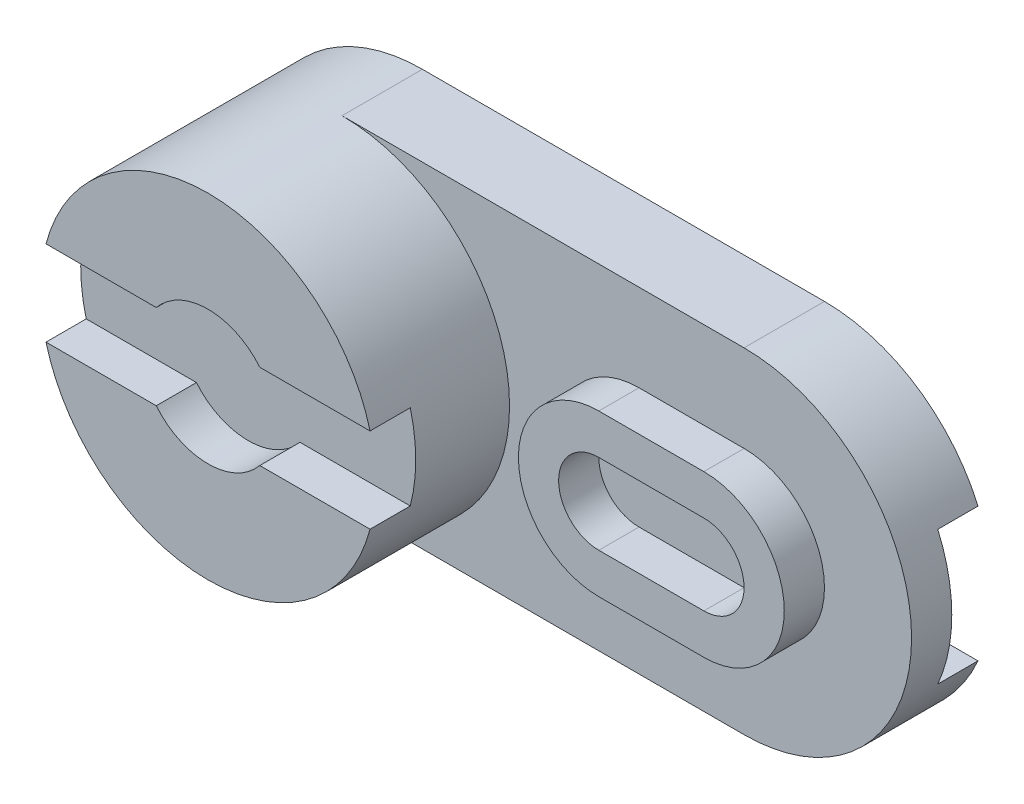
ISO-10303-21;
HEADER;
FILE_DESCRIPTION(('STEP AP214'),'2;1');
FILE_NAME('part.step','',(''),(''),'','','');
FILE_SCHEMA(('AUTOMOTIVE_DESIGN { 1 0 10303 214 1 1 1 1 }'));
ENDSEC;
DATA;
#1=APPLICATION_CONTEXT('core data for automotive mechanical design processes');
#2=APPLICATION_PROTOCOL_DEFINITION('international standard','automotive_design',2000,#1);
#3=PRODUCT_CONTEXT('',#1,'mechanical');
#4=PRODUCT('Part','Part','',(#3));
#5=PRODUCT_RELATED_PRODUCT_CATEGORY('part','',(#4));
#6=PRODUCT_DEFINITION_FORMATION('','',#4);
#7=PRODUCT_DEFINITION_CONTEXT('part definition',#1,'design');
#8=PRODUCT_DEFINITION('design','',#6,#7);
#9=PRODUCT_DEFINITION_SHAPE('','',#8);
#10=(LENGTH_UNIT() NAMED_UNIT(*) SI_UNIT(.MILLI.,.METRE.));
#11=(NAMED_UNIT(*) PLANE_ANGLE_UNIT() SI_UNIT($,.RADIAN.));
#12=(NAMED_UNIT(*) SI_UNIT($,.STERADIAN.) SOLID_ANGLE_UNIT());
#13=UNCERTAINTY_MEASURE_WITH_UNIT(LENGTH_MEASURE(1.E-05),#10,'distance_accuracy_value','');
#14=(GEOMETRIC_REPRESENTATION_CONTEXT(3) GLOBAL_UNCERTAINTY_ASSIGNED_CONTEXT((#13)) GLOBAL_UNIT_ASSIGNED_CONTEXT((#10,
#11,#12)) REPRESENTATION_CONTEXT('',''));
#15=CARTESIAN_POINT('',(0.,0.,0.));
#16=DIRECTION('',(0.,0.,1.));
#17=DIRECTION('',(1.,0.,0.));
#18=AXIS2_PLACEMENT_3D('',#15,#16,#17);
#19=CARTESIAN_POINT('',(0.,0.,12.));
#20=DIRECTION('',(0.,0.,1.));
#21=DIRECTION('',(1.,0.,0.));
#22=AXIS2_PLACEMENT_3D('',#19,#20,#21);
#23=PLANE('',#22);
#24=CARTESIAN_POINT('',(0.,0.,12.));
#25=DIRECTION('',(0.,0.,1.));
#26=DIRECTION('',(1.,0.,0.));
#27=AXIS2_PLACEMENT_3D('',#24,#25,#26);
#28=CIRCLE('',#27,25.);
#29=CARTESIAN_POINT('',(0.,-25.,12.));
#30=VERTEX_POINT('',#29);
#31=CARTESIAN_POINT('',(0.,25.,12.));
#32=VERTEX_POINT('',#31);
#33=EDGE_CURVE('E348',#30,#32,#28,.T.);
#34=ORIENTED_EDGE('',*,*,#33,.F.);
#35=DIRECTION('',(1.,0.,0.));
#36=VECTOR('',#35,1.);
#37=CARTESIAN_POINT('',(0.,-25.,12.));
#38=LINE('',#37,#36);
#39=CARTESIAN_POINT('',(60.,-25.,12.));
#40=VERTEX_POINT('',#39);
#41=EDGE_CURVE('E353',#30,#40,#38,.T.);
#42=ORIENTED_EDGE('',*,*,#41,.T.);
#43=CARTESIAN_POINT('',(60.,0.,12.));
#44=DIRECTION('',(0.,0.,1.));
#45=DIRECTION('',(1.,0.,0.));
#46=AXIS2_PLACEMENT_3D('',#43,#44,#45);
#47=CIRCLE('',#46,25.);
#48=CARTESIAN_POINT('',(60.,25.,12.));
#49=VERTEX_POINT('',#48);
#50=EDGE_CURVE('E359',#40,#49,#47,.T.);
#51=ORIENTED_EDGE('',*,*,#50,.T.);
#52=DIRECTION('',(-1.,0.,0.));
#53=VECTOR('',#52,1.);
#54=CARTESIAN_POINT('',(0.,25.,12.));
#55=LINE('',#54,#53);
#56=EDGE_CURVE('E356',#49,#32,#55,.T.);
#57=ORIENTED_EDGE('',*,*,#56,.T.);
#58=EDGE_LOOP('',(#34,#42,#51,#57));
#59=FACE_BOUND('',#58,.T.);
#60=DIRECTION('',(1.,0.,0.));
#61=VECTOR('',#60,1.);
#62=CARTESIAN_POINT('',(44.3230167016828,-12.,12.));
#63=LINE('',#62,#61);
#64=CARTESIAN_POINT('',(44.3230167016828,-12.,12.));
#65=VERTEX_POINT('',#64);
#66=CARTESIAN_POINT('',(60.,-12.,12.));
#67=VERTEX_POINT('',#66);
#68=EDGE_CURVE('E276',#65,#67,#63,.T.);
#69=ORIENTED_EDGE('',*,*,#68,.F.);
#70=CARTESIAN_POINT('',(44.3230167016828,0.,12.));
#71=DIRECTION('',(0.,0.,1.));
#72=DIRECTION('',(1.,0.,0.));
#73=AXIS2_PLACEMENT_3D('',#70,#71,#72);
#74=CIRCLE('',#73,12.);
#75=CARTESIAN_POINT('',(44.3230167016828,12.,12.));
#76=VERTEX_POINT('',#75);
#77=EDGE_CURVE('E264',#76,#65,#74,.T.);
#78=ORIENTED_EDGE('',*,*,#77,.F.);
#79=DIRECTION('',(-1.,0.,0.));
#80=VECTOR('',#79,1.);
#81=CARTESIAN_POINT('',(44.3230167016828,12.,12.));
#82=LINE('',#81,#80);
#83=CARTESIAN_POINT('',(60.,12.,12.));
#84=VERTEX_POINT('',#83);
#85=EDGE_CURVE('E269',#84,#76,#82,.T.);
#86=ORIENTED_EDGE('',*,*,#85,.F.);
#87=CARTESIAN_POINT('',(60.,0.,12.));
#88=DIRECTION('',(0.,0.,1.));
#89=DIRECTION('',(1.,0.,0.));
#90=AXIS2_PLACEMENT_3D('',#87,#88,#89);
#91=CIRCLE('',#90,12.);
#92=EDGE_CURVE('E282',#67,#84,#91,.T.);
#93=ORIENTED_EDGE('',*,*,#92,.F.);
#94=EDGE_LOOP('',(#69,#78,#86,#93));
#95=FACE_BOUND('',#94,.T.);
#96=ADVANCED_FACE('F39',(#59,#95),#23,.T.);
#97=CARTESIAN_POINT('',(0.,0.,12.));
#98=DIRECTION('',(0.,0.,-1.));
#99=DIRECTION('',(-1.,0.,0.));
#100=AXIS2_PLACEMENT_3D('',#97,#98,#99);
#101=CYLINDRICAL_SURFACE('',#100,25.);
#102=CARTESIAN_POINT('',(0.,0.,0.));
#103=DIRECTION('',(0.,0.,1.));
#104=DIRECTION('',(1.,0.,0.));
#105=AXIS2_PLACEMENT_3D('',#102,#103,#104);
#106=CIRCLE('',#105,25.);
#107=CARTESIAN_POINT('',(0.,25.,0.));
#108=VERTEX_POINT('',#107);
#109=CARTESIAN_POINT('',(0.,-25.,0.));
#110=VERTEX_POINT('',#109);
#111=EDGE_CURVE('E349',#108,#110,#106,.T.);
#112=ORIENTED_EDGE('',*,*,#111,.T.);
#113=DIRECTION('',(0.,0.,-1.));
#114=VECTOR('',#113,1.);
#115=CARTESIAN_POINT('',(0.,-25.,12.));
#116=LINE('',#115,#114);
#117=EDGE_CURVE('E351',#30,#110,#116,.T.);
#118=ORIENTED_EDGE('',*,*,#117,.F.);
#119=ORIENTED_EDGE('',*,*,#33,.T.);
#120=DIRECTION('',(0.,0.,-1.));
#121=VECTOR('',#120,1.);
#122=CARTESIAN_POINT('',(0.,25.,12.));
#123=LINE('',#122,#121);
#124=EDGE_CURVE('E361',#32,#108,#123,.T.);
#125=ORIENTED_EDGE('',*,*,#124,.T.);
#126=EDGE_LOOP('',(#112,#118,#119,#125));
#127=FACE_BOUND('',#126,.T.);
#128=DIRECTION('',(0.,0.,1.));
#129=VECTOR('',#128,1.);
#130=CARTESIAN_POINT('',(-24.1806910636993,-6.34776966200989,26.));
#131=LINE('',#130,#129);
#132=CARTESIAN_POINT('',(-24.1806910636993,-6.34776966200989,26.));
#133=VERTEX_POINT('',#132);
#134=CARTESIAN_POINT('',(-24.1806910636993,-6.34776966200989,32.));
#135=VERTEX_POINT('',#134);
#136=EDGE_CURVE('E330',#133,#135,#131,.T.);
#137=ORIENTED_EDGE('',*,*,#136,.F.);
#138=CARTESIAN_POINT('',(0.,0.,26.));
#139=DIRECTION('',(0.,0.,1.));
#140=DIRECTION('',(1.,0.,0.));
#141=AXIS2_PLACEMENT_3D('',#138,#139,#140);
#142=CIRCLE('',#141,25.);
#143=CARTESIAN_POINT('',(-24.1806910636993,6.34776966200989,26.));
#144=VERTEX_POINT('',#143);
#145=EDGE_CURVE('E313',#144,#133,#142,.T.);
#146=ORIENTED_EDGE('',*,*,#145,.F.);
#147=DIRECTION('',(0.,0.,1.));
#148=VECTOR('',#147,1.);
#149=CARTESIAN_POINT('',(-24.1806910636993,6.34776966200989,26.));
#150=LINE('',#149,#148);
#151=CARTESIAN_POINT('',(-24.1806910636993,6.34776966200989,32.));
#152=VERTEX_POINT('',#151);
#153=EDGE_CURVE('E329',#144,#152,#150,.T.);
#154=ORIENTED_EDGE('',*,*,#153,.T.);
#155=CARTESIAN_POINT('',(0.,0.,32.));
#156=DIRECTION('',(0.,0.,1.));
#157=DIRECTION('',(1.,0.,0.));
#158=AXIS2_PLACEMENT_3D('',#155,#156,#157);
#159=CIRCLE('',#158,25.);
#160=CARTESIAN_POINT('',(24.1806910636993,6.34776966200989,32.));
#161=VERTEX_POINT('',#160);
#162=EDGE_CURVE('E347',#161,#152,#159,.T.);
#163=ORIENTED_EDGE('',*,*,#162,.F.);
#164=DIRECTION('',(0.,0.,1.));
#165=VECTOR('',#164,1.);
#166=CARTESIAN_POINT('',(24.1806910636993,6.34776966200989,26.));
#167=LINE('',#166,#165);
#168=CARTESIAN_POINT('',(24.1806910636993,6.34776966200989,26.));
#169=VERTEX_POINT('',#168);
#170=EDGE_CURVE('E339',#169,#161,#167,.T.);
#171=ORIENTED_EDGE('',*,*,#170,.F.);
#172=CARTESIAN_POINT('',(0.,0.,26.));
#173=DIRECTION('',(0.,0.,1.));
#174=DIRECTION('',(1.,0.,0.));
#175=AXIS2_PLACEMENT_3D('',#172,#173,#174);
#176=CIRCLE('',#175,25.);
#177=CARTESIAN_POINT('',(24.1806910636993,-6.34776966200989,26.));
#178=VERTEX_POINT('',#177);
#179=EDGE_CURVE('E302',#178,#169,#176,.T.);
#180=ORIENTED_EDGE('',*,*,#179,.F.);
#181=DIRECTION('',(0.,0.,1.));
#182=VECTOR('',#181,1.);
#183=CARTESIAN_POINT('',(24.1806910636993,-6.34776966200989,26.));
#184=LINE('',#183,#182);
#185=CARTESIAN_POINT('',(24.1806910636993,-6.34776966200989,32.));
#186=VERTEX_POINT('',#185);
#187=EDGE_CURVE('E336',#178,#186,#184,.T.);
#188=ORIENTED_EDGE('',*,*,#187,.T.);
#189=EDGE_CURVE('E328',#135,#186,#159,.T.);
#190=ORIENTED_EDGE('',*,*,#189,.F.);
#191=EDGE_LOOP('',(#137,#146,#154,#163,#171,#180,#188,#190));
#192=FACE_BOUND('',#191,.T.);
#193=ADVANCED_FACE('F41',(#127,#192),#101,.T.);
#194=CARTESIAN_POINT('',(0.,0.,32.));
#195=DIRECTION('',(0.,0.,1.));
#196=DIRECTION('',(1.,0.,0.));
#197=AXIS2_PLACEMENT_3D('',#194,#195,#196);
#198=PLANE('',#197);
#199=CARTESIAN_POINT('',(0.,0.,32.));
#200=DIRECTION('',(0.,0.,1.));
#201=DIRECTION('',(1.,0.,0.));
#202=AXIS2_PLACEMENT_3D('',#199,#200,#201);
#203=CIRCLE('',#202,10.);
#204=CARTESIAN_POINT('',(-7.72695414235563,-6.34776966200989,32.));
#205=VERTEX_POINT('',#204);
#206=CARTESIAN_POINT('',(7.72695414235563,-6.34776966200989,32.));
#207=VERTEX_POINT('',#206);
#208=EDGE_CURVE('E320',#205,#207,#203,.T.);
#209=ORIENTED_EDGE('',*,*,#208,.F.);
#210=DIRECTION('',(-1.,0.,0.));
#211=VECTOR('',#210,1.);
#212=CARTESIAN_POINT('',(0.,-6.34776966200989,32.));
#213=LINE('',#212,#211);
#214=EDGE_CURVE('E295',#205,#135,#213,.T.);
#215=ORIENTED_EDGE('',*,*,#214,.T.);
#216=ORIENTED_EDGE('',*,*,#189,.T.);
#217=DIRECTION('',(1.,0.,0.));
#218=VECTOR('',#217,1.);
#219=CARTESIAN_POINT('',(0.,-6.34776966200989,32.));
#220=LINE('',#219,#218);
#221=EDGE_CURVE('E319',#207,#186,#220,.T.);
#222=ORIENTED_EDGE('',*,*,#221,.F.);
#223=EDGE_LOOP('',(#209,#215,#216,#222));
#224=FACE_BOUND('',#223,.T.);
#225=ADVANCED_FACE('F427',(#224),#198,.T.);
#226=CARTESIAN_POINT('',(0.,-25.,12.));
#227=DIRECTION('',(0.,1.,0.));
#228=DIRECTION('',(-1.,0.,0.));
#229=AXIS2_PLACEMENT_3D('',#226,#227,#228);
#230=PLANE('',#229);
#231=DIRECTION('',(1.,0.,0.));
#232=VECTOR('',#231,1.);
#233=CARTESIAN_POINT('',(0.,-25.,0.));
#234=LINE('',#233,#232);
#235=CARTESIAN_POINT('',(60.,-25.,0.));
#236=VERTEX_POINT('',#235);
#237=EDGE_CURVE('E368',#110,#236,#234,.T.);
#238=ORIENTED_EDGE('',*,*,#237,.T.);
#239=DIRECTION('',(0.,0.,-1.));
#240=VECTOR('',#239,1.);
#241=CARTESIAN_POINT('',(60.,-25.,12.));
#242=LINE('',#241,#240);
#243=EDGE_CURVE('E381',#40,#236,#242,.T.);
#244=ORIENTED_EDGE('',*,*,#243,.F.);
#245=ORIENTED_EDGE('',*,*,#41,.F.);
#246=ORIENTED_EDGE('',*,*,#117,.T.);
#247=EDGE_LOOP('',(#238,#244,#245,#246));
#248=FACE_BOUND('',#247,.T.);
#249=ADVANCED_FACE('F402',(#248),#230,.F.);
#250=CARTESIAN_POINT('',(60.,0.,12.));
#251=DIRECTION('',(0.,0.,-1.));
#252=DIRECTION('',(-1.,0.,0.));
#253=AXIS2_PLACEMENT_3D('',#250,#251,#252);
#254=CYLINDRICAL_SURFACE('',#253,25.);
#255=CARTESIAN_POINT('',(60.,0.,6.));
#256=DIRECTION('',(0.,0.,-1.));
#257=DIRECTION('',(-1.,0.,0.));
#258=AXIS2_PLACEMENT_3D('',#255,#256,#257);
#259=CIRCLE('',#258,25.);
#260=CARTESIAN_POINT('',(82.9128784747792,10.,6.));
#261=VERTEX_POINT('',#260);
#262=CARTESIAN_POINT('',(82.9128784747792,-10.,6.));
#263=VERTEX_POINT('',#262);
#264=EDGE_CURVE('E225',#261,#263,#259,.T.);
#265=ORIENTED_EDGE('',*,*,#264,.F.);
#266=DIRECTION('',(0.,0.,-1.));
#267=VECTOR('',#266,1.);
#268=CARTESIAN_POINT('',(82.9128784747792,10.,6.));
#269=LINE('',#268,#267);
#270=CARTESIAN_POINT('',(82.9128784747792,10.,-6.E-06));
#271=VERTEX_POINT('',#270);
#272=EDGE_CURVE('E218',#261,#271,#269,.T.);
#273=ORIENTED_EDGE('',*,*,#272,.T.);
#274=CARTESIAN_POINT('',(60.,0.,0.));
#275=DIRECTION('',(0.,0.,1.));
#276=DIRECTION('',(1.,0.,0.));
#277=AXIS2_PLACEMENT_3D('',#274,#275,#276);
#278=CIRCLE('',#277,25.);
#279=CARTESIAN_POINT('',(60.,25.,0.));
#280=VERTEX_POINT('',#279);
#281=EDGE_CURVE('E366',#271,#280,#278,.T.);
#282=ORIENTED_EDGE('',*,*,#281,.T.);
#283=DIRECTION('',(0.,0.,-1.));
#284=VECTOR('',#283,1.);
#285=CARTESIAN_POINT('',(60.,25.,12.));
#286=LINE('',#285,#284);
#287=EDGE_CURVE('E383',#49,#280,#286,.T.);
#288=ORIENTED_EDGE('',*,*,#287,.F.);
#289=ORIENTED_EDGE('',*,*,#50,.F.);
#290=ORIENTED_EDGE('',*,*,#243,.T.);
#291=CARTESIAN_POINT('',(82.9128784747792,-10.,0.));
#292=VERTEX_POINT('',#291);
#293=EDGE_CURVE('E376',#236,#292,#278,.T.);
#294=ORIENTED_EDGE('',*,*,#293,.T.);
#295=DIRECTION('',(0.,0.,-1.));
#296=VECTOR('',#295,1.);
#297=CARTESIAN_POINT('',(82.9128784747792,-10.,6.));
#298=LINE('',#297,#296);
#299=EDGE_CURVE('E54',#263,#292,#298,.T.);
#300=ORIENTED_EDGE('',*,*,#299,.F.);
#301=EDGE_LOOP('',(#265,#273,#282,#288,#289,#290,#294,#300));
#302=FACE_BOUND('',#301,.T.);
#303=ADVANCED_FACE('F410',(#302),#254,.T.);
#304=CARTESIAN_POINT('',(0.,25.,12.));
#305=DIRECTION('',(0.,-1.,0.));
#306=DIRECTION('',(1.,0.,0.));
#307=AXIS2_PLACEMENT_3D('',#304,#305,#306);
#308=PLANE('',#307);
#309=DIRECTION('',(-1.,0.,0.));
#310=VECTOR('',#309,1.);
#311=CARTESIAN_POINT('',(0.,25.,0.));
#312=LINE('',#311,#310);
#313=EDGE_CURVE('E357',#280,#108,#312,.T.);
#314=ORIENTED_EDGE('',*,*,#313,.T.);
#315=ORIENTED_EDGE('',*,*,#124,.F.);
#316=ORIENTED_EDGE('',*,*,#56,.F.);
#317=ORIENTED_EDGE('',*,*,#287,.T.);
#318=EDGE_LOOP('',(#314,#315,#316,#317));
#319=FACE_BOUND('',#318,.T.);
#320=ADVANCED_FACE('F407',(#319),#308,.F.);
#321=CARTESIAN_POINT('',(0.,0.,0.));
#322=DIRECTION('',(0.,0.,1.));
#323=DIRECTION('',(1.,0.,0.));
#324=AXIS2_PLACEMENT_3D('',#321,#322,#323);
#325=PLANE('',#324);
#326=ORIENTED_EDGE('',*,*,#281,.F.);
#327=DIRECTION('',(-1.,0.,0.));
#328=VECTOR('',#327,1.);
#329=CARTESIAN_POINT('',(0.,10.,0.));
#330=LINE('',#329,#328);
#331=CARTESIAN_POINT('',(60.,10.,0.));
#332=VERTEX_POINT('',#331);
#333=EDGE_CURVE('E11',#271,#332,#330,.T.);
#334=ORIENTED_EDGE('',*,*,#333,.T.);
#335=DIRECTION('',(0.,-1.,0.));
#336=VECTOR('',#335,1.);
#337=CARTESIAN_POINT('',(60.,0.,0.));
#338=LINE('',#337,#336);
#339=CARTESIAN_POINT('',(60.,-10.,0.));
#340=VERTEX_POINT('',#339);
#341=EDGE_CURVE('E48',#332,#340,#338,.T.);
#342=ORIENTED_EDGE('',*,*,#341,.T.);
#343=DIRECTION('',(-1.,0.,0.));
#344=VECTOR('',#343,1.);
#345=CARTESIAN_POINT('',(0.,-10.,0.));
#346=LINE('',#345,#344);
#347=EDGE_CURVE('E355',#292,#340,#346,.T.);
#348=ORIENTED_EDGE('',*,*,#347,.F.);
#349=ORIENTED_EDGE('',*,*,#293,.F.);
#350=ORIENTED_EDGE('',*,*,#237,.F.);
#351=ORIENTED_EDGE('',*,*,#111,.F.);
#352=ORIENTED_EDGE('',*,*,#313,.F.);
#353=EDGE_LOOP('',(#326,#334,#342,#348,#349,#350,#351,#352));
#354=FACE_BOUND('',#353,.T.);
#355=ADVANCED_FACE('F398',(#354),#325,.F.);
#356=DIRECTION('',(-1.,0.,0.));
#357=VECTOR('',#356,1.);
#358=CARTESIAN_POINT('',(0.,6.34776966200989,32.));
#359=LINE('',#358,#357);
#360=CARTESIAN_POINT('',(-7.72695414235563,6.34776966200989,32.));
#361=VERTEX_POINT('',#360);
#362=EDGE_CURVE('E297',#361,#152,#359,.T.);
#363=ORIENTED_EDGE('',*,*,#362,.F.);
#364=CARTESIAN_POINT('',(7.72695414235563,6.34776966200989,32.));
#365=VERTEX_POINT('',#364);
#366=EDGE_CURVE('E321',#365,#361,#203,.T.);
#367=ORIENTED_EDGE('',*,*,#366,.F.);
#368=DIRECTION('',(1.,0.,0.));
#369=VECTOR('',#368,1.);
#370=CARTESIAN_POINT('',(0.,6.34776966200989,32.));
#371=LINE('',#370,#369);
#372=EDGE_CURVE('E323',#365,#161,#371,.T.);
#373=ORIENTED_EDGE('',*,*,#372,.T.);
#374=ORIENTED_EDGE('',*,*,#162,.T.);
#375=EDGE_LOOP('',(#363,#367,#373,#374));
#376=FACE_BOUND('',#375,.T.);
#377=ADVANCED_FACE('F506',(#376),#198,.T.);
#378=CARTESIAN_POINT('',(0.,-6.34776966200989,26.));
#379=DIRECTION('',(0.,1.,0.));
#380=DIRECTION('',(-1.,0.,0.));
#381=AXIS2_PLACEMENT_3D('',#378,#379,#380);
#382=PLANE('',#381);
#383=ORIENTED_EDGE('',*,*,#214,.F.);
#384=DIRECTION('',(0.,0.,1.));
#385=VECTOR('',#384,1.);
#386=CARTESIAN_POINT('',(-7.72695414235563,-6.34776966200989,26.));
#387=LINE('',#386,#385);
#388=CARTESIAN_POINT('',(-7.72695414235563,-6.34776966200989,26.));
#389=VERTEX_POINT('',#388);
#390=EDGE_CURVE('E314',#389,#205,#387,.T.);
#391=ORIENTED_EDGE('',*,*,#390,.F.);
#392=DIRECTION('',(-1.,0.,0.));
#393=VECTOR('',#392,1.);
#394=CARTESIAN_POINT('',(0.,-6.34776966200989,26.));
#395=LINE('',#394,#393);
#396=EDGE_CURVE('E291',#389,#133,#395,.T.);
#397=ORIENTED_EDGE('',*,*,#396,.T.);
#398=ORIENTED_EDGE('',*,*,#136,.T.);
#399=EDGE_LOOP('',(#383,#391,#397,#398));
#400=FACE_BOUND('',#399,.T.);
#401=ADVANCED_FACE('F497',(#400),#382,.T.);
#402=CARTESIAN_POINT('',(0.,6.34776966200989,26.));
#403=DIRECTION('',(0.,1.,0.));
#404=DIRECTION('',(-1.,0.,0.));
#405=AXIS2_PLACEMENT_3D('',#402,#403,#404);
#406=PLANE('',#405);
#407=ORIENTED_EDGE('',*,*,#362,.T.);
#408=ORIENTED_EDGE('',*,*,#153,.F.);
#409=DIRECTION('',(-1.,0.,0.));
#410=VECTOR('',#409,1.);
#411=CARTESIAN_POINT('',(0.,6.34776966200989,26.));
#412=LINE('',#411,#410);
#413=CARTESIAN_POINT('',(-7.72695414235563,6.34776966200989,26.));
#414=VERTEX_POINT('',#413);
#415=EDGE_CURVE('E306',#414,#144,#412,.T.);
#416=ORIENTED_EDGE('',*,*,#415,.F.);
#417=DIRECTION('',(0.,0.,1.));
#418=VECTOR('',#417,1.);
#419=CARTESIAN_POINT('',(-7.72695414235563,6.34776966200989,26.));
#420=LINE('',#419,#418);
#421=EDGE_CURVE('E334',#414,#361,#420,.T.);
#422=ORIENTED_EDGE('',*,*,#421,.T.);
#423=EDGE_LOOP('',(#407,#408,#416,#422));
#424=FACE_BOUND('',#423,.T.);
#425=ADVANCED_FACE('F495',(#424),#406,.F.);
#426=CARTESIAN_POINT('',(0.,0.,26.));
#427=DIRECTION('',(0.,0.,1.));
#428=DIRECTION('',(1.,0.,0.));
#429=AXIS2_PLACEMENT_3D('',#426,#427,#428);
#430=CYLINDRICAL_SURFACE('',#429,10.);
#431=ORIENTED_EDGE('',*,*,#366,.T.);
#432=ORIENTED_EDGE('',*,*,#421,.F.);
#433=CARTESIAN_POINT('',(0.,0.,26.));
#434=DIRECTION('',(0.,0.,1.));
#435=DIRECTION('',(1.,0.,0.));
#436=AXIS2_PLACEMENT_3D('',#433,#434,#435);
#437=CIRCLE('',#436,10.);
#438=CARTESIAN_POINT('',(7.72695414235563,6.34776966200989,26.));
#439=VERTEX_POINT('',#438);
#440=EDGE_CURVE('E298',#439,#414,#437,.T.);
#441=ORIENTED_EDGE('',*,*,#440,.F.);
#442=DIRECTION('',(0.,0.,1.));
#443=VECTOR('',#442,1.);
#444=CARTESIAN_POINT('',(7.72695414235563,6.34776966200989,26.));
#445=LINE('',#444,#443);
#446=EDGE_CURVE('E333',#439,#365,#445,.T.);
#447=ORIENTED_EDGE('',*,*,#446,.T.);
#448=EDGE_LOOP('',(#431,#432,#441,#447));
#449=FACE_BOUND('',#448,.T.);
#450=ADVANCED_FACE('F494',(#449),#430,.F.);
#451=CARTESIAN_POINT('',(0.,6.34776966200989,26.));
#452=DIRECTION('',(0.,-1.,0.));
#453=DIRECTION('',(0.,0.,-1.));
#454=AXIS2_PLACEMENT_3D('',#451,#452,#453);
#455=PLANE('',#454);
#456=ORIENTED_EDGE('',*,*,#372,.F.);
#457=ORIENTED_EDGE('',*,*,#446,.F.);
#458=DIRECTION('',(1.,0.,0.));
#459=VECTOR('',#458,1.);
#460=CARTESIAN_POINT('',(0.,6.34776966200989,26.));
#461=LINE('',#460,#459);
#462=EDGE_CURVE('E308',#439,#169,#461,.T.);
#463=ORIENTED_EDGE('',*,*,#462,.T.);
#464=ORIENTED_EDGE('',*,*,#170,.T.);
#465=EDGE_LOOP('',(#456,#457,#463,#464));
#466=FACE_BOUND('',#465,.T.);
#467=ADVANCED_FACE('F498',(#466),#455,.T.);
#468=CARTESIAN_POINT('',(0.,-6.34776966200989,26.));
#469=DIRECTION('',(0.,-1.,0.));
#470=DIRECTION('',(0.,0.,-1.));
#471=AXIS2_PLACEMENT_3D('',#468,#469,#470);
#472=PLANE('',#471);
#473=ORIENTED_EDGE('',*,*,#221,.T.);
#474=ORIENTED_EDGE('',*,*,#187,.F.);
#475=DIRECTION('',(1.,0.,0.));
#476=VECTOR('',#475,1.);
#477=CARTESIAN_POINT('',(0.,-6.34776966200989,26.));
#478=LINE('',#477,#476);
#479=CARTESIAN_POINT('',(7.72695414235563,-6.34776966200989,26.));
#480=VERTEX_POINT('',#479);
#481=EDGE_CURVE('E296',#480,#178,#478,.T.);
#482=ORIENTED_EDGE('',*,*,#481,.F.);
#483=DIRECTION('',(0.,0.,1.));
#484=VECTOR('',#483,1.);
#485=CARTESIAN_POINT('',(7.72695414235563,-6.34776966200989,26.));
#486=LINE('',#485,#484);
#487=EDGE_CURVE('E344',#480,#207,#486,.T.);
#488=ORIENTED_EDGE('',*,*,#487,.T.);
#489=EDGE_LOOP('',(#473,#474,#482,#488));
#490=FACE_BOUND('',#489,.T.);
#491=ADVANCED_FACE('F501',(#490),#472,.F.);
#492=ORIENTED_EDGE('',*,*,#208,.T.);
#493=ORIENTED_EDGE('',*,*,#487,.F.);
#494=EDGE_CURVE('E293',#389,#480,#437,.T.);
#495=ORIENTED_EDGE('',*,*,#494,.F.);
#496=ORIENTED_EDGE('',*,*,#390,.T.);
#497=EDGE_LOOP('',(#492,#493,#495,#496));
#498=FACE_BOUND('',#497,.T.);
#499=ADVANCED_FACE('F489',(#498),#430,.F.);
#500=CARTESIAN_POINT('',(0.,0.,26.));
#501=DIRECTION('',(0.,0.,1.));
#502=DIRECTION('',(1.,0.,0.));
#503=AXIS2_PLACEMENT_3D('',#500,#501,#502);
#504=PLANE('',#503);
#505=ORIENTED_EDGE('',*,*,#396,.F.);
#506=ORIENTED_EDGE('',*,*,#494,.T.);
#507=ORIENTED_EDGE('',*,*,#481,.T.);
#508=ORIENTED_EDGE('',*,*,#179,.T.);
#509=ORIENTED_EDGE('',*,*,#462,.F.);
#510=ORIENTED_EDGE('',*,*,#440,.T.);
#511=ORIENTED_EDGE('',*,*,#415,.T.);
#512=ORIENTED_EDGE('',*,*,#145,.T.);
#513=EDGE_LOOP('',(#505,#506,#507,#508,#509,#510,#511,#512));
#514=FACE_BOUND('',#513,.T.);
#515=ADVANCED_FACE('F475',(#514),#504,.T.);
#516=CARTESIAN_POINT('',(44.3230167016828,0.,18.));
#517=DIRECTION('',(0.,0.,1.));
#518=DIRECTION('',(1.,0.,0.));
#519=AXIS2_PLACEMENT_3D('',#516,#517,#518);
#520=PLANE('',#519);
#521=CARTESIAN_POINT('',(44.3230167016828,0.,18.));
#522=DIRECTION('',(0.,0.,1.));
#523=DIRECTION('',(1.,0.,0.));
#524=AXIS2_PLACEMENT_3D('',#521,#522,#523);
#525=CIRCLE('',#524,12.);
#526=CARTESIAN_POINT('',(44.3230167016828,12.,18.));
#527=VERTEX_POINT('',#526);
#528=CARTESIAN_POINT('',(44.3230167016828,-12.,18.));
#529=VERTEX_POINT('',#528);
#530=EDGE_CURVE('E266',#527,#529,#525,.T.);
#531=ORIENTED_EDGE('',*,*,#530,.T.);
#532=DIRECTION('',(1.,0.,0.));
#533=VECTOR('',#532,1.);
#534=CARTESIAN_POINT('',(44.3230167016828,-12.,18.));
#535=LINE('',#534,#533);
#536=CARTESIAN_POINT('',(60.,-12.,18.));
#537=VERTEX_POINT('',#536);
#538=EDGE_CURVE('E267',#529,#537,#535,.T.);
#539=ORIENTED_EDGE('',*,*,#538,.T.);
#540=CARTESIAN_POINT('',(60.,0.,18.));
#541=DIRECTION('',(0.,0.,1.));
#542=DIRECTION('',(1.,0.,0.));
#543=AXIS2_PLACEMENT_3D('',#540,#541,#542);
#544=CIRCLE('',#543,12.);
#545=CARTESIAN_POINT('',(60.,12.,18.));
#546=VERTEX_POINT('',#545);
#547=EDGE_CURVE('E275',#537,#546,#544,.T.);
#548=ORIENTED_EDGE('',*,*,#547,.T.);
#549=DIRECTION('',(-1.,0.,0.));
#550=VECTOR('',#549,1.);
#551=CARTESIAN_POINT('',(44.3230167016828,12.,18.));
#552=LINE('',#551,#550);
#553=EDGE_CURVE('E273',#546,#527,#552,.T.);
#554=ORIENTED_EDGE('',*,*,#553,.T.);
#555=EDGE_LOOP('',(#531,#539,#548,#554));
#556=FACE_BOUND('',#555,.T.);
#557=DIRECTION('',(1.,0.,0.));
#558=VECTOR('',#557,1.);
#559=CARTESIAN_POINT('',(44.3230167016828,-6.,18.));
#560=LINE('',#559,#558);
#561=CARTESIAN_POINT('',(44.3230167016828,-6.,18.));
#562=VERTEX_POINT('',#561);
#563=CARTESIAN_POINT('',(60.,-6.,18.));
#564=VERTEX_POINT('',#563);
#565=EDGE_CURVE('E239',#562,#564,#560,.T.);
#566=ORIENTED_EDGE('',*,*,#565,.F.);
#567=CARTESIAN_POINT('',(44.3230167016828,0.,18.));
#568=DIRECTION('',(0.,0.,1.));
#569=DIRECTION('',(1.,0.,0.));
#570=AXIS2_PLACEMENT_3D('',#567,#568,#569);
#571=CIRCLE('',#570,5.99999999999999);
#572=CARTESIAN_POINT('',(44.3230167016828,5.99999999999999,18.));
#573=VERTEX_POINT('',#572);
#574=EDGE_CURVE('E240',#573,#562,#571,.T.);
#575=ORIENTED_EDGE('',*,*,#574,.F.);
#576=DIRECTION('',(-1.,0.,0.));
#577=VECTOR('',#576,1.);
#578=CARTESIAN_POINT('',(44.3230167016828,5.99999999999999,18.));
#579=LINE('',#578,#577);
#580=CARTESIAN_POINT('',(60.,6.,18.));
#581=VERTEX_POINT('',#580);
#582=EDGE_CURVE('E243',#581,#573,#579,.T.);
#583=ORIENTED_EDGE('',*,*,#582,.F.);
#584=CARTESIAN_POINT('',(60.,0.,18.));
#585=DIRECTION('',(0.,0.,1.));
#586=DIRECTION('',(1.,0.,0.));
#587=AXIS2_PLACEMENT_3D('',#584,#585,#586);
#588=CIRCLE('',#587,6.);
#589=EDGE_CURVE('E244',#564,#581,#588,.T.);
#590=ORIENTED_EDGE('',*,*,#589,.F.);
#591=EDGE_LOOP('',(#566,#575,#583,#590));
#592=FACE_BOUND('',#591,.T.);
#593=ADVANCED_FACE('F459',(#556,#592),#520,.T.);
#594=CARTESIAN_POINT('',(44.3230167016828,0.,18.));
#595=DIRECTION('',(0.,0.,-1.));
#596=DIRECTION('',(-1.,0.,0.));
#597=AXIS2_PLACEMENT_3D('',#594,#595,#596);
#598=CYLINDRICAL_SURFACE('',#597,12.);
#599=ORIENTED_EDGE('',*,*,#77,.T.);
#600=DIRECTION('',(0.,0.,-1.));
#601=VECTOR('',#600,1.);
#602=CARTESIAN_POINT('',(44.3230167016828,-12.,18.));
#603=LINE('',#602,#601);
#604=EDGE_CURVE('E286',#529,#65,#603,.T.);
#605=ORIENTED_EDGE('',*,*,#604,.F.);
#606=ORIENTED_EDGE('',*,*,#530,.F.);
#607=DIRECTION('',(0.,0.,-1.));
#608=VECTOR('',#607,1.);
#609=CARTESIAN_POINT('',(44.3230167016828,12.,18.));
#610=LINE('',#609,#608);
#611=EDGE_CURVE('E277',#527,#76,#610,.T.);
#612=ORIENTED_EDGE('',*,*,#611,.T.);
#613=EDGE_LOOP('',(#599,#605,#606,#612));
#614=FACE_BOUND('',#613,.T.);
#615=ADVANCED_FACE('F471',(#614),#598,.T.);
#616=CARTESIAN_POINT('',(44.3230167016828,-12.,18.));
#617=DIRECTION('',(0.,1.,0.));
#618=DIRECTION('',(-1.,0.,0.));
#619=AXIS2_PLACEMENT_3D('',#616,#617,#618);
#620=PLANE('',#619);
#621=ORIENTED_EDGE('',*,*,#68,.T.);
#622=DIRECTION('',(0.,0.,-1.));
#623=VECTOR('',#622,1.);
#624=CARTESIAN_POINT('',(60.,-12.,18.));
#625=LINE('',#624,#623);
#626=EDGE_CURVE('E289',#537,#67,#625,.T.);
#627=ORIENTED_EDGE('',*,*,#626,.F.);
#628=ORIENTED_EDGE('',*,*,#538,.F.);
#629=ORIENTED_EDGE('',*,*,#604,.T.);
#630=EDGE_LOOP('',(#621,#627,#628,#629));
#631=FACE_BOUND('',#630,.T.);
#632=ADVANCED_FACE('F481',(#631),#620,.F.);
#633=CARTESIAN_POINT('',(60.,0.,18.));
#634=DIRECTION('',(0.,0.,-1.));
#635=DIRECTION('',(-1.,0.,0.));
#636=AXIS2_PLACEMENT_3D('',#633,#634,#635);
#637=CYLINDRICAL_SURFACE('',#636,12.);
#638=ORIENTED_EDGE('',*,*,#92,.T.);
#639=DIRECTION('',(0.,0.,-1.));
#640=VECTOR('',#639,1.);
#641=CARTESIAN_POINT('',(60.,12.,18.));
#642=LINE('',#641,#640);
#643=EDGE_CURVE('E65',#546,#84,#642,.T.);
#644=ORIENTED_EDGE('',*,*,#643,.F.);
#645=ORIENTED_EDGE('',*,*,#547,.F.);
#646=ORIENTED_EDGE('',*,*,#626,.T.);
#647=EDGE_LOOP('',(#638,#644,#645,#646));
#648=FACE_BOUND('',#647,.T.);
#649=ADVANCED_FACE('F476',(#648),#637,.T.);
#650=CARTESIAN_POINT('',(44.3230167016828,12.,18.));
#651=DIRECTION('',(0.,-1.,0.));
#652=DIRECTION('',(1.,0.,0.));
#653=AXIS2_PLACEMENT_3D('',#650,#651,#652);
#654=PLANE('',#653);
#655=ORIENTED_EDGE('',*,*,#85,.T.);
#656=ORIENTED_EDGE('',*,*,#611,.F.);
#657=ORIENTED_EDGE('',*,*,#553,.F.);
#658=ORIENTED_EDGE('',*,*,#643,.T.);
#659=EDGE_LOOP('',(#655,#656,#657,#658));
#660=FACE_BOUND('',#659,.T.);
#661=ADVANCED_FACE('F473',(#660),#654,.F.);
#662=CARTESIAN_POINT('',(44.3230167016828,0.,18.));
#663=DIRECTION('',(0.,0.,-1.));
#664=DIRECTION('',(-1.,0.,0.));
#665=AXIS2_PLACEMENT_3D('',#662,#663,#664);
#666=CYLINDRICAL_SURFACE('',#665,5.99999999999999);
#667=CARTESIAN_POINT('',(44.3230167016828,0.,12.));
#668=DIRECTION('',(0.,0.,1.));
#669=DIRECTION('',(1.,0.,0.));
#670=AXIS2_PLACEMENT_3D('',#667,#668,#669);
#671=CIRCLE('',#670,5.99999999999999);
#672=CARTESIAN_POINT('',(44.3230167016828,5.99999999999999,12.));
#673=VERTEX_POINT('',#672);
#674=CARTESIAN_POINT('',(44.3230167016828,-6.,12.));
#675=VERTEX_POINT('',#674);
#676=EDGE_CURVE('E215',#673,#675,#671,.T.);
#677=ORIENTED_EDGE('',*,*,#676,.F.);
#678=DIRECTION('',(0.,0.,-1.));
#679=VECTOR('',#678,1.);
#680=CARTESIAN_POINT('',(44.3230167016828,5.99999999999999,18.));
#681=LINE('',#680,#679);
#682=EDGE_CURVE('E249',#573,#673,#681,.T.);
#683=ORIENTED_EDGE('',*,*,#682,.F.);
#684=ORIENTED_EDGE('',*,*,#574,.T.);
#685=DIRECTION('',(0.,0.,-1.));
#686=VECTOR('',#685,1.);
#687=CARTESIAN_POINT('',(44.3230167016828,-6.,18.));
#688=LINE('',#687,#686);
#689=EDGE_CURVE('E265',#562,#675,#688,.T.);
#690=ORIENTED_EDGE('',*,*,#689,.T.);
#691=EDGE_LOOP('',(#677,#683,#684,#690));
#692=FACE_BOUND('',#691,.T.);
#693=ADVANCED_FACE('F451',(#692),#666,.F.);
#694=CARTESIAN_POINT('',(44.3230167016828,-6.,18.));
#695=DIRECTION('',(0.,1.,0.));
#696=DIRECTION('',(-1.,0.,0.));
#697=AXIS2_PLACEMENT_3D('',#694,#695,#696);
#698=PLANE('',#697);
#699=DIRECTION('',(1.,0.,0.));
#700=VECTOR('',#699,1.);
#701=CARTESIAN_POINT('',(44.3230167016828,-6.,12.));
#702=LINE('',#701,#700);
#703=CARTESIAN_POINT('',(60.,-6.,12.));
#704=VERTEX_POINT('',#703);
#705=EDGE_CURVE('E250',#675,#704,#702,.T.);
#706=ORIENTED_EDGE('',*,*,#705,.F.);
#707=ORIENTED_EDGE('',*,*,#689,.F.);
#708=ORIENTED_EDGE('',*,*,#565,.T.);
#709=DIRECTION('',(0.,0.,-1.));
#710=VECTOR('',#709,1.);
#711=CARTESIAN_POINT('',(60.,-6.,18.));
#712=LINE('',#711,#710);
#713=EDGE_CURVE('E259',#564,#704,#712,.T.);
#714=ORIENTED_EDGE('',*,*,#713,.T.);
#715=EDGE_LOOP('',(#706,#707,#708,#714));
#716=FACE_BOUND('',#715,.T.);
#717=ADVANCED_FACE('F453',(#716),#698,.T.);
#718=CARTESIAN_POINT('',(60.,0.,18.));
#719=DIRECTION('',(0.,0.,-1.));
#720=DIRECTION('',(-1.,0.,0.));
#721=AXIS2_PLACEMENT_3D('',#718,#719,#720);
#722=CYLINDRICAL_SURFACE('',#721,6.);
#723=CARTESIAN_POINT('',(60.,0.,12.));
#724=DIRECTION('',(0.,0.,1.));
#725=DIRECTION('',(1.,0.,0.));
#726=AXIS2_PLACEMENT_3D('',#723,#724,#725);
#727=CIRCLE('',#726,6.);
#728=CARTESIAN_POINT('',(60.,6.,12.));
#729=VERTEX_POINT('',#728);
#730=EDGE_CURVE('E253',#704,#729,#727,.T.);
#731=ORIENTED_EDGE('',*,*,#730,.F.);
#732=ORIENTED_EDGE('',*,*,#713,.F.);
#733=ORIENTED_EDGE('',*,*,#589,.T.);
#734=DIRECTION('',(0.,0.,-1.));
#735=VECTOR('',#734,1.);
#736=CARTESIAN_POINT('',(60.,6.,18.));
#737=LINE('',#736,#735);
#738=EDGE_CURVE('E258',#581,#729,#737,.T.);
#739=ORIENTED_EDGE('',*,*,#738,.T.);
#740=EDGE_LOOP('',(#731,#732,#733,#739));
#741=FACE_BOUND('',#740,.T.);
#742=ADVANCED_FACE('F442',(#741),#722,.F.);
#743=CARTESIAN_POINT('',(44.3230167016828,5.99999999999999,18.));
#744=DIRECTION('',(0.,-1.,0.));
#745=DIRECTION('',(1.,0.,0.));
#746=AXIS2_PLACEMENT_3D('',#743,#744,#745);
#747=PLANE('',#746);
#748=DIRECTION('',(-1.,0.,0.));
#749=VECTOR('',#748,1.);
#750=CARTESIAN_POINT('',(44.3230167016828,5.99999999999999,12.));
#751=LINE('',#750,#749);
#752=EDGE_CURVE('E238',#729,#673,#751,.T.);
#753=ORIENTED_EDGE('',*,*,#752,.F.);
#754=ORIENTED_EDGE('',*,*,#738,.F.);
#755=ORIENTED_EDGE('',*,*,#582,.T.);
#756=ORIENTED_EDGE('',*,*,#682,.T.);
#757=EDGE_LOOP('',(#753,#754,#755,#756));
#758=FACE_BOUND('',#757,.T.);
#759=ADVANCED_FACE('F433',(#758),#747,.T.);
#760=ORIENTED_EDGE('',*,*,#676,.T.);
#761=ORIENTED_EDGE('',*,*,#705,.T.);
#762=ORIENTED_EDGE('',*,*,#730,.T.);
#763=ORIENTED_EDGE('',*,*,#752,.T.);
#764=EDGE_LOOP('',(#760,#761,#762,#763));
#765=FACE_BOUND('',#764,.T.);
#766=ADVANCED_FACE('F421',(#765),#23,.T.);
#767=CARTESIAN_POINT('',(60.,0.,-1.2E-05));
#768=DIRECTION('',(-1.,0.,0.));
#769=DIRECTION('',(0.,0.,1.));
#770=AXIS2_PLACEMENT_3D('',#767,#768,#769);
#771=PLANE('',#770);
#772=DIRECTION('',(0.,0.,1.));
#773=VECTOR('',#772,1.);
#774=CARTESIAN_POINT('',(60.,10.,-1.2E-05));
#775=LINE('',#774,#773);
#776=CARTESIAN_POINT('',(60.,10.,6.));
#777=VERTEX_POINT('',#776);
#778=EDGE_CURVE('E201',#332,#777,#775,.T.);
#779=ORIENTED_EDGE('',*,*,#778,.T.);
#780=DIRECTION('',(0.,-1.,0.));
#781=VECTOR('',#780,1.);
#782=CARTESIAN_POINT('',(60.,0.,6.));
#783=LINE('',#782,#781);
#784=CARTESIAN_POINT('',(60.,-10.,6.));
#785=VERTEX_POINT('',#784);
#786=EDGE_CURVE('E208',#777,#785,#783,.T.);
#787=ORIENTED_EDGE('',*,*,#786,.T.);
#788=DIRECTION('',(0.,0.,1.));
#789=VECTOR('',#788,1.);
#790=CARTESIAN_POINT('',(60.,-10.,-1.2E-05));
#791=LINE('',#790,#789);
#792=EDGE_CURVE('E213',#340,#785,#791,.T.);
#793=ORIENTED_EDGE('',*,*,#792,.F.);
#794=ORIENTED_EDGE('',*,*,#341,.F.);
#795=EDGE_LOOP('',(#779,#787,#793,#794));
#796=FACE_BOUND('',#795,.T.);
#797=ADVANCED_FACE('F202',(#796),#771,.F.);
#798=CARTESIAN_POINT('',(0.,10.,-1.2E-05));
#799=DIRECTION('',(0.,1.,0.));
#800=DIRECTION('',(0.,0.,1.));
#801=AXIS2_PLACEMENT_3D('',#798,#799,#800);
#802=PLANE('',#801);
#803=ORIENTED_EDGE('',*,*,#272,.F.);
#804=DIRECTION('',(-1.,0.,0.));
#805=VECTOR('',#804,1.);
#806=CARTESIAN_POINT('',(0.,10.,6.));
#807=LINE('',#806,#805);
#808=EDGE_CURVE('E216',#261,#777,#807,.T.);
#809=ORIENTED_EDGE('',*,*,#808,.T.);
#810=ORIENTED_EDGE('',*,*,#778,.F.);
#811=ORIENTED_EDGE('',*,*,#333,.F.);
#812=EDGE_LOOP('',(#803,#809,#810,#811));
#813=FACE_BOUND('',#812,.T.);
#814=ADVANCED_FACE('F220',(#813),#802,.F.);
#815=CARTESIAN_POINT('',(0.,-10.,-1.2E-05));
#816=DIRECTION('',(0.,1.,0.));
#817=DIRECTION('',(0.,0.,1.));
#818=AXIS2_PLACEMENT_3D('',#815,#816,#817);
#819=PLANE('',#818);
#820=ORIENTED_EDGE('',*,*,#347,.T.);
#821=ORIENTED_EDGE('',*,*,#792,.T.);
#822=DIRECTION('',(-1.,0.,0.));
#823=VECTOR('',#822,1.);
#824=CARTESIAN_POINT('',(0.,-10.,6.));
#825=LINE('',#824,#823);
#826=EDGE_CURVE('E223',#263,#785,#825,.T.);
#827=ORIENTED_EDGE('',*,*,#826,.F.);
#828=ORIENTED_EDGE('',*,*,#299,.T.);
#829=EDGE_LOOP('',(#820,#821,#827,#828));
#830=FACE_BOUND('',#829,.T.);
#831=ADVANCED_FACE('F414',(#830),#819,.T.);
#832=CARTESIAN_POINT('',(0.,0.,6.));
#833=DIRECTION('',(0.,0.,-1.));
#834=DIRECTION('',(-1.,0.,0.));
#835=AXIS2_PLACEMENT_3D('',#832,#833,#834);
#836=PLANE('',#835);
#837=ORIENTED_EDGE('',*,*,#786,.F.);
#838=ORIENTED_EDGE('',*,*,#808,.F.);
#839=ORIENTED_EDGE('',*,*,#264,.T.);
#840=ORIENTED_EDGE('',*,*,#826,.T.);
#841=EDGE_LOOP('',(#837,#838,#839,#840));
#842=FACE_BOUND('',#841,.T.);
#843=ADVANCED_FACE('F221',(#842),#836,.T.);
#844=CLOSED_SHELL('',(#96,#193,#225,#249,#303,#320,#355,#377,#401,#425,#450,#467,#491,#499,#515,
#593,#615,#632,#649,#661,#693,#717,#742,#759,#766,#797,#814,#831,#843));
#845=MANIFOLD_SOLID_BREP('B2',#844);
#846=ADVANCED_BREP_SHAPE_REPRESENTATION('',(#18,#845),#14);
#847=SHAPE_DEFINITION_REPRESENTATION(#9,#846);
ENDSEC;
END-ISO-10303-21;
